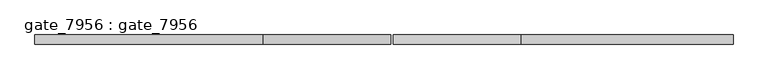
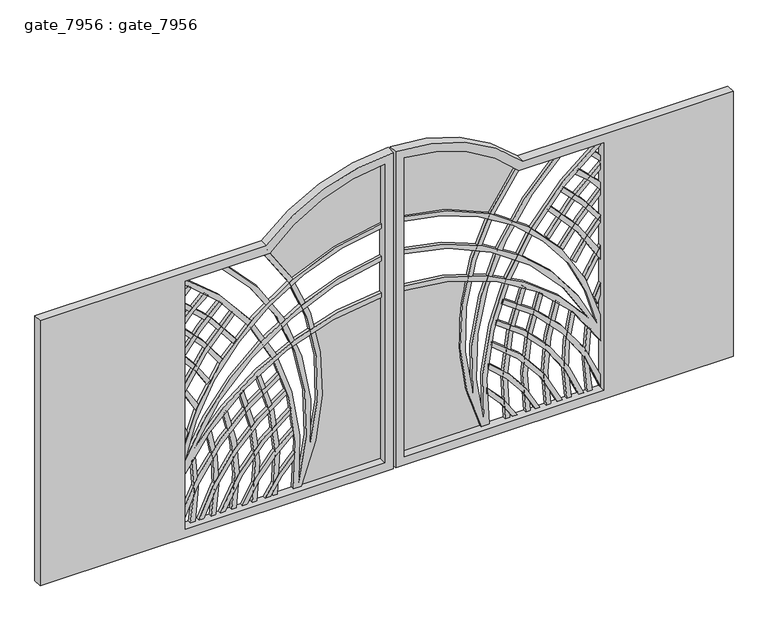
"""IFC4 building model written with IfcOpenShell, lengths in millimetres: proxy geometry, gate_7956 : gate_7956."""

from ifc_helpers import new_model, si_unit, point, frame, frame_2d, origin, place, context, project, spatial, polyline, circle_curve, trimmed, segment, composite_curve, outline, extrude, source, transform, mapped, element, save


def gate_7956_gate_7956_2a423054(model_context):
    return source(origin(), model_context, "Body", "SweptSolid", [
        extrude(outline(composite_curve([segment(polyline([(1574.8, -714.375), (1574.8, -1986.4480277), (0.0, -1986.4480277), (0.0, 0.0), (1879.3736556, 0.0)]), True, "CONTINUOUS"), segment(trimmed(circle_curve(frame_2d((881.859553, 3.175)), 997.5191555), [point((1879.3736556, 0.0))], [point((1574.8, -714.375))], False, "CARTESIAN"), True, "CONTINUOUS")], self_intersect=False), holes=[composite_curve([segment(polyline([(1827.2147875, -47.625), (50.8, -47.625), (50.8, -1171.575), (1524.0, -1171.575), (1524.0, -692.4777911)]), True, "CONTINUOUS"), segment(trimmed(circle_curve(frame_2d((881.859553, 3.175)), 946.7191555), [point((1524.0, -692.4777911))], [point((1827.2147875, -47.625))], True, "CARTESIAN"), True, "CONTINUOUS")], self_intersect=False)]), frame((0.0, -50.8, 0.0), z_axis=(0.0, 1.0, 0.0), x_axis=(0.0, 0.0, 1.0)), (0.0, 0.0, 1.0), 50.8),
        extrude(outline(composite_curve([segment(trimmed(circle_curve(frame_2d((188.1193765, 65.6258097)), 1270.1981582), [point((1453.2587424, -47.625))], [point((475.7606767, -1171.575))], False, "CARTESIAN"), True, "CONTINUOUS"), segment(polyline([(475.7606767, -1171.575), (325.438753, -1171.575)]), True, "CONTINUOUS"), segment(trimmed(circle_curve(frame_2d((-306.470048, -9.2092819)), 1323.0278891), [point((325.438753, -1171.575))], [point((1016.0, -47.625))], True, "CARTESIAN"), True, "CONTINUOUS"), segment(polyline([(1016.0, -47.625), (1042.85139, -47.625)]), True, "CONTINUOUS"), segment(trimmed(circle_curve(frame_2d((-321.9912288, -1.7370637)), 1365.6138095), [point((1042.85139, -47.625))], [point((487.9033995, -1101.269586))], False, "CARTESIAN"), True, "CONTINUOUS"), segment(trimmed(circle_curve(frame_2d((-94.5667128, 101.7568292)), 1336.6166195), [point((487.9033995, -1101.269586))], [point((1233.6761327, -47.625))], True, "CARTESIAN"), True, "CONTINUOUS"), segment(polyline([(1233.6761327, -47.625), (1259.2332506, -47.625)]), True, "CONTINUOUS"), segment(trimmed(circle_curve(frame_2d((-94.5667128, 101.7568292)), 1362.0166195), [point((1259.2332506, -47.625))], [point((428.8390935, -1155.6753295))], False, "CARTESIAN"), True, "CONTINUOUS"), segment(trimmed(circle_curve(frame_2d((188.1193765, 65.6258097)), 1244.7981582), [point((428.8390935, -1155.6753295))], [point((1427.7550927, -47.625))], True, "CARTESIAN"), True, "CONTINUOUS"), segment(polyline([(1427.7550927, -47.625), (1453.2587424, -47.625)]), True, "CONTINUOUS")], self_intersect=False)), frame((0.0, -19.05, 0.0), z_axis=(0.0, 1.0, 0.0), x_axis=(0.0, 0.0, 1.0)), (0.0, 0.0, 1.0), 19.05),
        extrude(outline(composite_curve([segment(trimmed(circle_curve(frame_2d((625.1927136, -1831.8247988)), 1451.1947292), [point((50.8, -499.1436094))], [point((1524.0, -692.4777911))], False, "CARTESIAN"), True, "CONTINUOUS"), segment(polyline([(1524.0, -692.4777911), (1524.0, -717.8616311), (1508.2761961, -712.4096154)]), True, "CONTINUOUS"), segment(trimmed(circle_curve(frame_2d((625.2005352, -1831.8604357)), 1425.8305516), [point((1508.2761961, -712.4096154))], [point((270.5135839, -450.849962))], True, "CARTESIAN"), True, "CONTINUOUS"), segment(trimmed(circle_curve(frame_2d((428.9211986, -1911.4736244)), 1469.1883662), [point((270.5135839, -450.849962))], [point((1524.0, -932.0263955))], False, "CARTESIAN"), True, "CONTINUOUS"), segment(polyline([(1524.0, -932.0263955), (1524.0, -970.5462776)]), True, "CONTINUOUS"), segment(trimmed(circle_curve(frame_2d((434.6192112, -1905.6521568)), 1435.6787622), [point((1524.0, -970.5462776))], [point((79.5169904, -514.5820935))], True, "CARTESIAN"), True, "CONTINUOUS"), segment(trimmed(circle_curve(frame_2d((251.9754674, -2051.8469137)), 1546.9082241), [point((79.5169904, -514.5820935))], [point((1524.0, -1171.575))], False, "CARTESIAN"), True, "CONTINUOUS"), segment(polyline([(1524.0, -1171.575), (1492.986601, -1171.575)]), True, "CONTINUOUS"), segment(trimmed(circle_curve(frame_2d((251.9754674, -2051.8469137)), 1521.5082241), [point((1492.986601, -1171.575))], [point((50.8, -543.6971508))], True, "CARTESIAN"), True, "CONTINUOUS"), segment(polyline([(50.8, -543.6971508), (50.8, -499.1436094)]), True, "CONTINUOUS")], self_intersect=False)), frame((0.0, -19.05, 0.0), z_axis=(0.0, 1.0, 0.0), x_axis=(0.0, 0.0, 1.0)), (0.0, 0.0, 1.0), 19.05),
        extrude(outline(composite_curve([segment(trimmed(circle_curve(frame_2d((-321.9912288, -1.7370636)), 1251.3138095), [point((766.023996, -619.8059275))], [point((122.1545272, -1171.575))], False, "CARTESIAN"), True, "CONTINUOUS"), segment(polyline([(122.1545272, -1171.575), (50.8, -1171.575)]), True, "CONTINUOUS"), segment(trimmed(circle_curve(frame_2d((-329.3476454, 3.2021804)), 1234.7524675), [point((50.8, -1171.575))], [point((741.6413557, -611.2864))], True, "CARTESIAN"), True, "CONTINUOUS"), segment(polyline([(741.6413557, -611.2864), (766.023996, -619.8059275)]), True, "CONTINUOUS")], self_intersect=False)), frame((0.0, -19.05, 0.0), z_axis=(0.0, 1.0, 0.0), x_axis=(0.0, 0.0, 1.0)), (0.0, 0.0, 1.0), 19.05),
        extrude(outline(composite_curve([segment(trimmed(circle_curve(frame_2d((-321.9912288, -1.7370637)), 1137.0138095), [point((654.3216834, -584.5007383))], [point((50.8, -1075.9005069))], False, "CARTESIAN"), True, "CONTINUOUS"), segment(polyline([(50.8, -1075.9005069), (50.8, -1048.9772277)]), True, "CONTINUOUS"), segment(trimmed(circle_curve(frame_2d((-321.9912288, -1.7370637)), 1111.6138095), [point((50.8, -1048.9772277))], [point((628.7552213, -577.7287729))], True, "CARTESIAN"), True, "CONTINUOUS"), segment(polyline([(628.7552213, -577.7287729), (654.3216834, -584.5007383)]), True, "CONTINUOUS")], self_intersect=False)), frame((0.0, -19.05, 0.0), z_axis=(0.0, 1.0, 0.0), x_axis=(0.0, 0.0, 1.0)), (0.0, 0.0, 1.0), 19.05),
        extrude(outline(composite_curve([segment(trimmed(circle_curve(frame_2d((-321.9912288, -1.7370637)), 1022.7138095), [point((536.7182406, -557.2202617))], [point((50.8, -954.0869132))], False, "CARTESIAN"), True, "CONTINUOUS"), segment(polyline([(50.8, -954.0869132), (50.8, -926.7568118)]), True, "CONTINUOUS"), segment(trimmed(circle_curve(frame_2d((-321.9912288, -1.7370637)), 997.3138095), [point((50.8, -926.7568118))], [point((510.8571668, -550.3702604))], True, "CARTESIAN"), True, "CONTINUOUS"), segment(polyline([(510.8571668, -550.3702604), (536.7182406, -557.2202617)]), True, "CONTINUOUS")], self_intersect=False)), frame((0.0, -19.05, 0.0), z_axis=(0.0, 1.0, 0.0), x_axis=(0.0, 0.0, 1.0)), (0.0, 0.0, 1.0), 19.05),
        extrude(outline(composite_curve([segment(trimmed(circle_curve(frame_2d((-321.9912288, -1.7370637)), 908.4138095), [point((410.7722159, -538.6480277))], [point((50.8, -830.134522))], False, "CARTESIAN"), True, "CONTINUOUS"), segment(polyline([(50.8, -830.134522), (50.8, -802.1994847)]), True, "CONTINUOUS"), segment(trimmed(circle_curve(frame_2d((-321.9912288, -1.7370637)), 883.0138095), [point((50.8, -802.1994847))], [point((379.0365912, -538.6480277))], True, "CARTESIAN"), True, "CONTINUOUS"), segment(polyline([(379.0365912, -538.6480277), (410.7722159, -538.6480277)]), True, "CONTINUOUS")], self_intersect=False)), frame((0.0, -19.05, 0.0), z_axis=(0.0, 1.0, 0.0), x_axis=(0.0, 0.0, 1.0)), (0.0, 0.0, 1.0), 19.05),
        extrude(outline(composite_curve([segment(trimmed(circle_curve(frame_2d((-321.9912288, -1.7370637)), 794.1138095), [point((270.5266887, -530.4517881))], [point((50.8, -702.9099683))], False, "CARTESIAN"), True, "CONTINUOUS"), segment(polyline([(50.8, -702.9099683), (50.8, -674.0075603)]), True, "CONTINUOUS"), segment(trimmed(circle_curve(frame_2d((-321.9912288, -1.7370637)), 768.7138095), [point((50.8, -674.0075603))], [point((236.0245963, -530.4517881))], True, "CARTESIAN"), True, "CONTINUOUS"), segment(polyline([(236.0245963, -530.4517881), (270.5266887, -530.4517881)]), True, "CONTINUOUS")], self_intersect=False)), frame((0.0, -19.05, 0.0), z_axis=(0.0, 1.0, 0.0), x_axis=(0.0, 0.0, 1.0)), (0.0, 0.0, 1.0), 19.05),
        extrude(outline(composite_curve([segment(polyline([(1210.9602193, -867.4506933), (1228.939295, -885.429769)]), True, "CONTINUOUS"), segment(trimmed(circle_curve(frame_2d((188.1193765, 65.6258097)), 1409.8981582), [point((1228.939295, -885.429769))], [point((864.245824, -1171.575))], False, "CARTESIAN"), True, "CONTINUOUS"), segment(polyline([(864.245824, -1171.575), (809.5445985, -1171.575)]), True, "CONTINUOUS"), segment(trimmed(circle_curve(frame_2d((188.1193765, 65.6258097)), 1384.4981582), [point((809.5445985, -1171.575))], [point((1210.9602193, -867.4506933))], True, "CARTESIAN"), True, "CONTINUOUS")], self_intersect=False)), frame((0.0, -19.05, 0.0), z_axis=(0.0, 1.0, 0.0), x_axis=(0.0, 0.0, 1.0)), (0.0, 0.0, 1.0), 19.05),
        extrude(outline(composite_curve([segment(polyline([(1295.7670706, -944.0833092), (1313.7464656, -962.0627043)]), True, "CONTINUOUS"), segment(trimmed(circle_curve(frame_2d((298.9547736, -40.580869)), 1370.7410225), [point((1313.7464656, -962.0627043))], [point((1073.4115036, -1171.575))], False, "CARTESIAN"), True, "CONTINUOUS"), segment(polyline([(1073.4115036, -1171.575), (1034.1276953, -1171.575)]), True, "CONTINUOUS"), segment(trimmed(circle_curve(frame_2d((188.1193765, 65.6258097)), 1498.7981582), [point((1034.1276953, -1171.575))], [point((1295.7670706, -944.0833092))], True, "CARTESIAN"), True, "CONTINUOUS")], self_intersect=False)), frame((0.0, -19.05, 0.0), z_axis=(0.0, 1.0, 0.0), x_axis=(0.0, 0.0, 1.0)), (0.0, 0.0, 1.0), 19.05),
        extrude(outline(composite_curve([segment(polyline([(1371.3808408, -1023.8325474), (1393.8084123, -1046.2601189)]), True, "CONTINUOUS"), segment(trimmed(circle_curve(frame_2d((157.0059526, 65.2274597)), 1662.854462), [point((1393.8084123, -1046.2601189))], [point((1268.4935312, -1171.575))], False, "CARTESIAN"), True, "CONTINUOUS"), segment(polyline([(1268.4935312, -1171.575), (1223.2134903, -1171.575)]), True, "CONTINUOUS"), segment(trimmed(circle_curve(frame_2d((881.0604584, -680.2699964)), 598.7063586), [point((1223.2134903, -1171.575))], [point((1371.3808408, -1023.8325474))], True, "CARTESIAN"), True, "CONTINUOUS")], self_intersect=False)), frame((0.0, -19.05, 0.0), z_axis=(0.0, 1.0, 0.0), x_axis=(0.0, 0.0, 1.0)), (0.0, 0.0, 1.0), 19.05),
        extrude(outline(composite_curve([segment(polyline([(1448.1437026, -1116.942791), (1466.2607278, -1135.0598162)]), True, "CONTINUOUS"), segment(trimmed(circle_curve(frame_2d((2369.5144168, -2074.828689)), 1303.469509), [point((1466.2607278, -1135.0598162))], [point((1429.745544, -1171.575))], True, "CARTESIAN"), True, "CONTINUOUS"), segment(polyline([(1429.745544, -1171.575), (1393.6228205, -1171.575)]), True, "CONTINUOUS"), segment(trimmed(circle_curve(frame_2d((2581.8039176, -2302.8138821)), 1640.5717686), [point((1393.6228205, -1171.575))], [point((1448.1437026, -1116.942791))], False, "CARTESIAN"), True, "CONTINUOUS")], self_intersect=False)), frame((0.0, -19.05, 0.0), z_axis=(0.0, 1.0, 0.0), x_axis=(0.0, 0.0, 1.0)), (0.0, 0.0, 1.0), 19.05),
        extrude(outline(composite_curve([segment(polyline([(50.8, -1123.3836365), (50.8, -1096.2682984)]), True, "CONTINUOUS"), segment(trimmed(circle_curve(frame_2d((249.227799, -2294.693819)), 1214.741668), [point((50.8, -1096.2682984))], [point((439.2593722, -1094.9082877))], False, "CARTESIAN"), True, "CONTINUOUS"), segment(polyline([(439.2593722, -1094.9082877), (417.7529701, -1116.4146899)]), True, "CONTINUOUS"), segment(trimmed(circle_curve(frame_2d((251.9754674, -2051.8469137)), 950.0082241), [point((417.7529701, -1116.4146899))], [point((50.8, -1123.3836365))], True, "CARTESIAN"), True, "CONTINUOUS")], self_intersect=False)), frame((0.0, -19.05, 0.0), z_axis=(0.0, 1.0, 0.0), x_axis=(0.0, 0.0, 1.0)), (0.0, 0.0, 1.0), 19.05),
        extrude(outline(composite_curve([segment(polyline([(50.8, -1006.7247069), (50.8, -980.869582)]), True, "CONTINUOUS"), segment(trimmed(circle_curve(frame_2d((251.9754674, -2051.8469137)), 1089.7082241), [point((50.8, -980.869582))], [point((559.4182819, -1006.4078053))], False, "CARTESIAN"), True, "CONTINUOUS"), segment(polyline([(559.4182819, -1006.4078053), (538.8861292, -1026.939958)]), True, "CONTINUOUS"), segment(trimmed(circle_curve(frame_2d((251.9754674, -2051.8469137)), 1064.3082241), [point((538.8861292, -1026.939958))], [point((50.8, -1006.7247069))], True, "CARTESIAN"), True, "CONTINUOUS")], self_intersect=False)), frame((0.0, -19.05, 0.0), z_axis=(0.0, 1.0, 0.0), x_axis=(0.0, 0.0, 1.0)), (0.0, 0.0, 1.0), 19.05),
        extrude(outline(composite_curve([segment(polyline([(50.8, -890.30598), (50.8, -864.7646777)]), True, "CONTINUOUS"), segment(trimmed(circle_curve(frame_2d((251.9754674, -2051.8469137)), 1204.0082241), [point((50.8, -864.7646777))], [point((656.0575932, -917.6716895))], False, "CARTESIAN"), True, "CONTINUOUS"), segment(polyline([(656.0575932, -917.6716895), (636.1282841, -937.6009986)]), True, "CONTINUOUS"), segment(trimmed(circle_curve(frame_2d((249.671635, -2074.7397377)), 1201.0134277), [point((636.1282841, -937.6009986))], [point((50.8, -890.30598))], True, "CARTESIAN"), True, "CONTINUOUS")], self_intersect=False)), frame((0.0, -19.05, 0.0), z_axis=(0.0, 1.0, 0.0), x_axis=(0.0, 0.0, 1.0)), (0.0, 0.0, 1.0), 19.05),
        extrude(outline(composite_curve([segment(polyline([(50.8, -774.6859578), (50.8, -748.9789216)]), True, "CONTINUOUS"), segment(trimmed(circle_curve(frame_2d((251.9754674, -2051.8469137)), 1318.3082241), [point((50.8, -748.9789216))], [point((737.9350335, -826.3756274))], False, "CARTESIAN"), True, "CONTINUOUS"), segment(polyline([(737.9350335, -826.3756274), (718.3335001, -845.9771607)]), True, "CONTINUOUS"), segment(trimmed(circle_curve(frame_2d((251.9754674, -2051.8469137)), 1292.9082241), [point((718.3335001, -845.9771607))], [point((50.8, -774.6859578))], True, "CARTESIAN"), True, "CONTINUOUS")], self_intersect=False)), frame((0.0, -19.05, 0.0), z_axis=(0.0, 1.0, 0.0), x_axis=(0.0, 0.0, 1.0)), (0.0, 0.0, 1.0), 19.05),
        extrude(outline(composite_curve([segment(polyline([(50.8, -659.0930168), (50.8, -633.4341547)]), True, "CONTINUOUS"), segment(trimmed(circle_curve(frame_2d((251.9754674, -2051.8469137)), 1432.6082241), [point((50.8, -633.4341547))], [point((808.380048, -731.7028813))], False, "CARTESIAN"), True, "CONTINUOUS"), segment(polyline([(808.380048, -731.7028813), (788.9599222, -751.1230071)]), True, "CONTINUOUS"), segment(trimmed(circle_curve(frame_2d((251.9754674, -2051.8469137)), 1407.2082241), [point((788.9599222, -751.1230071))], [point((50.8, -659.0930168))], True, "CARTESIAN"), True, "CONTINUOUS")], self_intersect=False)), frame((0.0, -19.05, 0.0), z_axis=(0.0, 1.0, 0.0), x_axis=(0.0, 0.0, 1.0)), (0.0, 0.0, 1.0), 19.05),
        extrude(outline(polyline([(553.3842288, -1150.9205103), (593.450224, -1138.1641492), (672.1451492, -1171.575), (609.2386529, -1171.575), (553.3842288, -1150.9205103)])), frame((0.0, -19.05, 0.0), z_axis=(0.0, 1.0, 0.0), x_axis=(0.0, 0.0, 1.0)), (0.0, 0.0, 1.0), 19.05),
        extrude(outline(composite_curve([segment(trimmed(circle_curve(frame_2d((251.9754673, -2051.8469137)), 1064.3082241), [point((850.2006371, -1171.575))], [point((711.3700205, -1091.7903318))], True, "CARTESIAN"), True, "CONTINUOUS"), segment(polyline([(711.3700205, -1091.7903318), (740.9012216, -1077.980588)]), True, "CONTINUOUS"), segment(trimmed(circle_curve(frame_2d((251.9754674, -2051.8469137)), 1089.7082241), [point((740.9012216, -1077.980588))], [point((894.3035545, -1171.575))], False, "CARTESIAN"), True, "CONTINUOUS"), segment(polyline([(894.3035545, -1171.575), (850.2006371, -1171.575)]), True, "CONTINUOUS")], self_intersect=False)), frame((0.0, -19.05, 0.0), z_axis=(0.0, 1.0, 0.0), x_axis=(0.0, 0.0, 1.0)), (0.0, 0.0, 1.0), 19.05),
        extrude(outline(composite_curve([segment(trimmed(circle_curve(frame_2d((436.5150762, -1780.3292563)), 853.0665783), [point((1034.1276953, -1171.575))], [point((842.2813497, -1029.9451424))], True, "CARTESIAN"), True, "CONTINUOUS"), segment(polyline([(842.2813497, -1029.9451424), (859.7363544, -1012.4901377)]), True, "CONTINUOUS"), segment(trimmed(circle_curve(frame_2d((251.9754673, -2051.8469137)), 1204.0082241), [point((859.7363544, -1012.4901377))], [point((1073.4115036, -1171.575))], False, "CARTESIAN"), True, "CONTINUOUS"), segment(polyline([(1073.4115036, -1171.575), (1034.1276953, -1171.575)]), True, "CONTINUOUS")], self_intersect=False)), frame((0.0, -19.05, 0.0), z_axis=(0.0, 1.0, 0.0), x_axis=(0.0, 0.0, 1.0)), (0.0, 0.0, 1.0), 19.05),
        extrude(outline(composite_curve([segment(polyline([(943.9740273, -959.7161207), (962.3717805, -941.3183675)]), True, "CONTINUOUS"), segment(trimmed(circle_curve(frame_2d((251.9754673, -2051.8469138)), 1318.3082242), [point((962.3717805, -941.3183675))], [point((1233.3306179, -1171.575))], False, "CARTESIAN"), True, "CONTINUOUS"), segment(polyline([(1233.3306179, -1171.575), (1198.9353576, -1171.575)]), True, "CONTINUOUS"), segment(trimmed(circle_curve(frame_2d((251.9754673, -2051.8469138)), 1292.9082241), [point((1198.9353576, -1171.575))], [point((943.9740273, -959.7161207))], True, "CARTESIAN"), True, "CONTINUOUS")], self_intersect=False)), frame((0.0, -19.05, 0.0), z_axis=(0.0, 1.0, 0.0), x_axis=(0.0, 0.0, 1.0)), (0.0, 0.0, 1.0), 19.05),
        extrude(outline(composite_curve([segment(polyline([(1035.0267606, -882.6310833), (1053.3289179, -864.3289261)]), True, "CONTINUOUS"), segment(trimmed(circle_curve(frame_2d((251.9754673, -2051.8469137)), 1432.6082241), [point((1053.3289179, -864.3289261))], [point((1382.2354736, -1171.575))], False, "CARTESIAN"), True, "CONTINUOUS"), segment(polyline([(1382.2354736, -1171.575), (1349.8626855, -1171.575)]), True, "CONTINUOUS"), segment(trimmed(circle_curve(frame_2d((251.9754674, -2051.8469137)), 1407.2082241), [point((1349.8626855, -1171.575))], [point((1035.0267606, -882.6310833))], True, "CARTESIAN"), True, "CONTINUOUS")], self_intersect=False)), frame((0.0, -19.05, 0.0), z_axis=(0.0, 1.0, 0.0), x_axis=(0.0, 0.0, 1.0)), (0.0, 0.0, 1.0), 19.05),
        extrude(outline(composite_curve([segment(trimmed(circle_curve(frame_2d((881.859553, 3.175)), 946.7191555), [point((1827.2147875, -47.625))], [point((1524.0, -692.4777911))], False, "CARTESIAN"), True, "CONTINUOUS"), segment(trimmed(circle_curve(frame_2d((625.1927137, -1831.8247988)), 1451.1947292), [point((1524.0, -692.4777911))], [point((1300.6036994, -547.3847876))], True, "CARTESIAN"), True, "CONTINUOUS"), segment(trimmed(circle_curve(frame_2d((188.1193765, 65.6258097)), 1270.1981582), [point((1300.6036994, -547.3847876))], [point((1453.2587424, -47.625))], True, "CARTESIAN"), True, "CONTINUOUS"), segment(polyline([(1453.2587424, -47.625), (1827.2147875, -47.625)]), True, "CONTINUOUS")], self_intersect=False)), frame((0.0, -6.35, 0.0), z_axis=(0.0, 1.0, 0.0), x_axis=(0.0, 0.0, 1.0)), (0.0, 0.0, 1.0), 6.35),
        extrude(outline(composite_curve([segment(trimmed(circle_curve(frame_2d((-306.470048, -9.2092819)), 1323.0278891), [point((1016.0, -47.625))], [point((951.8602911, -417.8748577))], False, "CARTESIAN"), True, "CONTINUOUS"), segment(trimmed(circle_curve(frame_2d((625.1927136, -1831.8247988)), 1451.1947292), [point((951.8602911, -417.8748577))], [point((50.8, -499.1436094))], True, "CARTESIAN"), True, "CONTINUOUS"), segment(polyline([(50.8, -499.1436094), (50.8, -47.625), (1016.0, -47.625)]), True, "CONTINUOUS")], self_intersect=False)), frame((0.0, -6.35, 0.0), z_axis=(0.0, 1.0, 0.0), x_axis=(0.0, 0.0, 1.0)), (0.0, 0.0, 1.0), 6.35),
        extrude(outline(composite_curve([segment(trimmed(circle_curve(frame_2d((881.859553, 9.525)), 997.5191555), [point((1574.8, 727.075))], [point((1879.3736556, 12.7))], False, "CARTESIAN"), True, "CONTINUOUS"), segment(polyline([(1879.3736556, 12.7), (0.0, 12.7), (0.0, 1910.3857812), (1574.8, 1910.3857812), (1574.8, 727.075)]), True, "CONTINUOUS")], self_intersect=False), holes=[composite_curve([segment(trimmed(circle_curve(frame_2d((881.859553, 9.525)), 946.7191555), [point((1827.2147875, 60.325))], [point((1524.0, 705.1777911))], True, "CARTESIAN"), True, "CONTINUOUS"), segment(polyline([(1524.0, 705.1777911), (1524.0, 1184.275), (50.8, 1184.275), (50.8, 60.325), (1827.2147875, 60.325)]), True, "CONTINUOUS")], self_intersect=False)]), frame((0.0, -50.8, 0.0), z_axis=(0.0, 1.0, 0.0), x_axis=(0.0, 0.0, 1.0)), (0.0, 0.0, 1.0), 50.8),
        extrude(outline(composite_curve([segment(polyline([(1453.2587424, 60.325), (1427.7550927, 60.325)]), True, "CONTINUOUS"), segment(trimmed(circle_curve(frame_2d((188.1193765, -52.9258097)), 1244.7981582), [point((1427.7550927, 60.325))], [point((428.8390935, 1168.3753295))], True, "CARTESIAN"), True, "CONTINUOUS"), segment(trimmed(circle_curve(frame_2d((-94.5667128, -89.0568292)), 1362.0166195), [point((428.8390935, 1168.3753295))], [point((1259.2332506, 60.325))], False, "CARTESIAN"), True, "CONTINUOUS"), segment(polyline([(1259.2332506, 60.325), (1233.6761327, 60.325)]), True, "CONTINUOUS"), segment(trimmed(circle_curve(frame_2d((-94.5667128, -89.0568292)), 1336.6166195), [point((1233.6761327, 60.325))], [point((487.9033995, 1113.969586))], True, "CARTESIAN"), True, "CONTINUOUS"), segment(trimmed(circle_curve(frame_2d((-321.9912288, 14.4370637)), 1365.6138095), [point((487.9033995, 1113.969586))], [point((1042.85139, 60.325))], False, "CARTESIAN"), True, "CONTINUOUS"), segment(polyline([(1042.85139, 60.325), (1016.0, 60.325)]), True, "CONTINUOUS"), segment(trimmed(circle_curve(frame_2d((-306.470048, 21.9092819)), 1323.0278891), [point((1016.0, 60.325))], [point((325.438753, 1184.275))], True, "CARTESIAN"), True, "CONTINUOUS"), segment(polyline([(325.438753, 1184.275), (475.7606767, 1184.275)]), True, "CONTINUOUS"), segment(trimmed(circle_curve(frame_2d((188.1193765, -52.9258097)), 1270.1981582), [point((475.7606767, 1184.275))], [point((1453.2587424, 60.325))], False, "CARTESIAN"), True, "CONTINUOUS")], self_intersect=False)), frame((0.0, -19.05, 0.0), z_axis=(0.0, 1.0, 0.0), x_axis=(0.0, 0.0, 1.0)), (0.0, 0.0, 1.0), 19.05),
        extrude(outline(composite_curve([segment(polyline([(50.8, 511.8436094), (50.8, 556.3971508)]), True, "CONTINUOUS"), segment(trimmed(circle_curve(frame_2d((251.9754674, 2064.5469137)), 1521.5082241), [point((50.8, 556.3971508))], [point((1492.986601, 1184.275))], True, "CARTESIAN"), True, "CONTINUOUS"), segment(polyline([(1492.986601, 1184.275), (1524.0, 1184.275)]), True, "CONTINUOUS"), segment(trimmed(circle_curve(frame_2d((251.9754674, 2064.5469137)), 1546.9082241), [point((1524.0, 1184.275))], [point((79.5169904, 527.2820935))], False, "CARTESIAN"), True, "CONTINUOUS"), segment(trimmed(circle_curve(frame_2d((434.6192112, 1918.3521568)), 1435.6787622), [point((79.5169904, 527.2820935))], [point((1524.0, 983.2462776))], True, "CARTESIAN"), True, "CONTINUOUS"), segment(polyline([(1524.0, 983.2462776), (1524.0, 944.7263955)]), True, "CONTINUOUS"), segment(trimmed(circle_curve(frame_2d((428.9211986, 1924.1736244)), 1469.1883662), [point((1524.0, 944.7263955))], [point((270.5135839, 463.549962))], False, "CARTESIAN"), True, "CONTINUOUS"), segment(trimmed(circle_curve(frame_2d((625.2005352, 1844.5604357)), 1425.8305516), [point((270.5135839, 463.549962))], [point((1508.2761961, 725.1096154))], True, "CARTESIAN"), True, "CONTINUOUS"), segment(polyline([(1508.2761961, 725.1096154), (1524.0, 730.5616311), (1524.0, 705.1777911)]), True, "CONTINUOUS"), segment(trimmed(circle_curve(frame_2d((625.1927136, 1844.5247988)), 1451.1947292), [point((1524.0, 705.1777911))], [point((50.8, 511.8436094))], False, "CARTESIAN"), True, "CONTINUOUS")], self_intersect=False)), frame((0.0, -19.05, 0.0), z_axis=(0.0, 1.0, 0.0), x_axis=(0.0, 0.0, 1.0)), (0.0, 0.0, 1.0), 19.05),
        extrude(outline(composite_curve([segment(polyline([(766.023996, 632.5059275), (741.6413557, 623.9864)]), True, "CONTINUOUS"), segment(trimmed(circle_curve(frame_2d((-329.3476454, 9.4978196)), 1234.7524675), [point((741.6413557, 623.9864))], [point((50.8, 1184.275))], True, "CARTESIAN"), True, "CONTINUOUS"), segment(polyline([(50.8, 1184.275), (122.1545272, 1184.275)]), True, "CONTINUOUS"), segment(trimmed(circle_curve(frame_2d((-321.9912288, 14.4370636)), 1251.3138095), [point((122.1545272, 1184.275))], [point((766.023996, 632.5059275))], False, "CARTESIAN"), True, "CONTINUOUS")], self_intersect=False)), frame((0.0, -19.05, 0.0), z_axis=(0.0, 1.0, 0.0), x_axis=(0.0, 0.0, 1.0)), (0.0, 0.0, 1.0), 19.05),
        extrude(outline(composite_curve([segment(polyline([(654.3216834, 597.2007383), (628.7552213, 590.4287729)]), True, "CONTINUOUS"), segment(trimmed(circle_curve(frame_2d((-321.9912288, 14.4370637)), 1111.6138095), [point((628.7552213, 590.4287729))], [point((50.8, 1061.6772277))], True, "CARTESIAN"), True, "CONTINUOUS"), segment(polyline([(50.8, 1061.6772277), (50.8, 1088.6005069)]), True, "CONTINUOUS"), segment(trimmed(circle_curve(frame_2d((-321.9912288, 14.4370637)), 1137.0138095), [point((50.8, 1088.6005069))], [point((654.3216834, 597.2007383))], False, "CARTESIAN"), True, "CONTINUOUS")], self_intersect=False)), frame((0.0, -19.05, 0.0), z_axis=(0.0, 1.0, 0.0), x_axis=(0.0, 0.0, 1.0)), (0.0, 0.0, 1.0), 19.05),
        extrude(outline(composite_curve([segment(polyline([(536.7182406, 569.9202617), (510.8571668, 563.0702604)]), True, "CONTINUOUS"), segment(trimmed(circle_curve(frame_2d((-321.9912288, 14.4370637)), 997.3138095), [point((510.8571668, 563.0702604))], [point((50.8, 939.4568118))], True, "CARTESIAN"), True, "CONTINUOUS"), segment(polyline([(50.8, 939.4568118), (50.8, 966.7869132)]), True, "CONTINUOUS"), segment(trimmed(circle_curve(frame_2d((-321.9912288, 14.4370637)), 1022.7138095), [point((50.8, 966.7869132))], [point((536.7182406, 569.9202617))], False, "CARTESIAN"), True, "CONTINUOUS")], self_intersect=False)), frame((0.0, -19.05, 0.0), z_axis=(0.0, 1.0, 0.0), x_axis=(0.0, 0.0, 1.0)), (0.0, 0.0, 1.0), 19.05),
        extrude(outline(composite_curve([segment(polyline([(410.7722159, 551.3480277), (379.0365912, 551.3480277)]), True, "CONTINUOUS"), segment(trimmed(circle_curve(frame_2d((-321.9912288, 14.4370637)), 883.0138095), [point((379.0365912, 551.3480277))], [point((50.8, 814.8994847))], True, "CARTESIAN"), True, "CONTINUOUS"), segment(polyline([(50.8, 814.8994847), (50.8, 842.834522)]), True, "CONTINUOUS"), segment(trimmed(circle_curve(frame_2d((-321.9912288, 14.4370637)), 908.4138095), [point((50.8, 842.834522))], [point((410.7722159, 551.3480277))], False, "CARTESIAN"), True, "CONTINUOUS")], self_intersect=False)), frame((0.0, -19.05, 0.0), z_axis=(0.0, 1.0, 0.0), x_axis=(0.0, 0.0, 1.0)), (0.0, 0.0, 1.0), 19.05),
        extrude(outline(composite_curve([segment(polyline([(270.5266887, 543.1517881), (236.0245963, 543.1517881)]), True, "CONTINUOUS"), segment(trimmed(circle_curve(frame_2d((-321.9912288, 14.4370637)), 768.7138095), [point((236.0245963, 543.1517881))], [point((50.8, 686.7075603))], True, "CARTESIAN"), True, "CONTINUOUS"), segment(polyline([(50.8, 686.7075603), (50.8, 715.6099683)]), True, "CONTINUOUS"), segment(trimmed(circle_curve(frame_2d((-321.9912288, 14.4370637)), 794.1138095), [point((50.8, 715.6099683))], [point((270.5266887, 543.1517881))], False, "CARTESIAN"), True, "CONTINUOUS")], self_intersect=False)), frame((0.0, -19.05, 0.0), z_axis=(0.0, 1.0, 0.0), x_axis=(0.0, 0.0, 1.0)), (0.0, 0.0, 1.0), 19.05),
        extrude(outline(composite_curve([segment(trimmed(circle_curve(frame_2d((188.1193765, -52.9258097)), 1384.4981582), [point((1210.9602193, 880.1506933))], [point((809.5445985, 1184.275))], True, "CARTESIAN"), True, "CONTINUOUS"), segment(polyline([(809.5445985, 1184.275), (864.245824, 1184.275)]), True, "CONTINUOUS"), segment(trimmed(circle_curve(frame_2d((188.1193765, -52.9258097)), 1409.8981582), [point((864.245824, 1184.275))], [point((1228.939295, 898.129769))], False, "CARTESIAN"), True, "CONTINUOUS"), segment(polyline([(1228.939295, 898.129769), (1210.9602193, 880.1506933)]), True, "CONTINUOUS")], self_intersect=False)), frame((0.0, -19.05, 0.0), z_axis=(0.0, 1.0, 0.0), x_axis=(0.0, 0.0, 1.0)), (0.0, 0.0, 1.0), 19.05),
        extrude(outline(composite_curve([segment(trimmed(circle_curve(frame_2d((188.1193765, -52.9258097)), 1498.7981582), [point((1295.7670706, 956.7833092))], [point((1034.1276953, 1184.275))], True, "CARTESIAN"), True, "CONTINUOUS"), segment(polyline([(1034.1276953, 1184.275), (1073.4115036, 1184.275)]), True, "CONTINUOUS"), segment(trimmed(circle_curve(frame_2d((298.9547736, 53.280869)), 1370.7410225), [point((1073.4115036, 1184.275))], [point((1313.7464656, 974.7627043))], False, "CARTESIAN"), True, "CONTINUOUS"), segment(polyline([(1313.7464656, 974.7627043), (1295.7670706, 956.7833092)]), True, "CONTINUOUS")], self_intersect=False)), frame((0.0, -19.05, 0.0), z_axis=(0.0, 1.0, 0.0), x_axis=(0.0, 0.0, 1.0)), (0.0, 0.0, 1.0), 19.05),
        extrude(outline(composite_curve([segment(trimmed(circle_curve(frame_2d((881.0604584, 692.9699964)), 598.7063586), [point((1371.3808408, 1036.5325474))], [point((1223.2134903, 1184.275))], True, "CARTESIAN"), True, "CONTINUOUS"), segment(polyline([(1223.2134903, 1184.275), (1268.4935312, 1184.275)]), True, "CONTINUOUS"), segment(trimmed(circle_curve(frame_2d((157.0059526, -52.5274597)), 1662.854462), [point((1268.4935312, 1184.275))], [point((1393.8084123, 1058.9601189))], False, "CARTESIAN"), True, "CONTINUOUS"), segment(polyline([(1393.8084123, 1058.9601189), (1371.3808408, 1036.5325474)]), True, "CONTINUOUS")], self_intersect=False)), frame((0.0, -19.05, 0.0), z_axis=(0.0, 1.0, 0.0), x_axis=(0.0, 0.0, 1.0)), (0.0, 0.0, 1.0), 19.05),
        extrude(outline(composite_curve([segment(trimmed(circle_curve(frame_2d((2581.8039176, 2315.5138821)), 1640.5717686), [point((1448.1437026, 1129.642791))], [point((1393.6228205, 1184.275))], False, "CARTESIAN"), True, "CONTINUOUS"), segment(polyline([(1393.6228205, 1184.275), (1429.745544, 1184.275)]), True, "CONTINUOUS"), segment(trimmed(circle_curve(frame_2d((2369.5144168, 2087.528689)), 1303.469509), [point((1429.745544, 1184.275))], [point((1466.2607278, 1147.7598162))], True, "CARTESIAN"), True, "CONTINUOUS"), segment(polyline([(1466.2607278, 1147.7598162), (1448.1437026, 1129.642791)]), True, "CONTINUOUS")], self_intersect=False)), frame((0.0, -19.05, 0.0), z_axis=(0.0, 1.0, 0.0), x_axis=(0.0, 0.0, 1.0)), (0.0, 0.0, 1.0), 19.05),
        extrude(outline(composite_curve([segment(trimmed(circle_curve(frame_2d((251.9754674, 2064.5469137)), 950.0082241), [point((50.8, 1136.0836365))], [point((417.7529701, 1129.1146899))], True, "CARTESIAN"), True, "CONTINUOUS"), segment(polyline([(417.7529701, 1129.1146899), (439.2593722, 1107.6082877)]), True, "CONTINUOUS"), segment(trimmed(circle_curve(frame_2d((249.227799, 2307.393819)), 1214.741668), [point((439.2593722, 1107.6082877))], [point((50.8, 1108.9682984))], False, "CARTESIAN"), True, "CONTINUOUS"), segment(polyline([(50.8, 1108.9682984), (50.8, 1136.0836365)]), True, "CONTINUOUS")], self_intersect=False)), frame((0.0, -19.05, 0.0), z_axis=(0.0, 1.0, 0.0), x_axis=(0.0, 0.0, 1.0)), (0.0, 0.0, 1.0), 19.05),
        extrude(outline(composite_curve([segment(trimmed(circle_curve(frame_2d((251.9754674, 2064.5469137)), 1064.3082241), [point((50.8, 1019.4247069))], [point((538.8861292, 1039.639958))], True, "CARTESIAN"), True, "CONTINUOUS"), segment(polyline([(538.8861292, 1039.639958), (559.4182819, 1019.1078053)]), True, "CONTINUOUS"), segment(trimmed(circle_curve(frame_2d((251.9754674, 2064.5469137)), 1089.7082241), [point((559.4182819, 1019.1078053))], [point((50.8, 993.569582))], False, "CARTESIAN"), True, "CONTINUOUS"), segment(polyline([(50.8, 993.569582), (50.8, 1019.4247069)]), True, "CONTINUOUS")], self_intersect=False)), frame((0.0, -19.05, 0.0), z_axis=(0.0, 1.0, 0.0), x_axis=(0.0, 0.0, 1.0)), (0.0, 0.0, 1.0), 19.05),
        extrude(outline(composite_curve([segment(trimmed(circle_curve(frame_2d((249.671635, 2087.4397377)), 1201.0134277), [point((50.8, 903.00598))], [point((636.1282841, 950.3009986))], True, "CARTESIAN"), True, "CONTINUOUS"), segment(polyline([(636.1282841, 950.3009986), (656.0575932, 930.3716895)]), True, "CONTINUOUS"), segment(trimmed(circle_curve(frame_2d((251.9754674, 2064.5469137)), 1204.0082241), [point((656.0575932, 930.3716895))], [point((50.8, 877.4646777))], False, "CARTESIAN"), True, "CONTINUOUS"), segment(polyline([(50.8, 877.4646777), (50.8, 903.00598)]), True, "CONTINUOUS")], self_intersect=False)), frame((0.0, -19.05, 0.0), z_axis=(0.0, 1.0, 0.0), x_axis=(0.0, 0.0, 1.0)), (0.0, 0.0, 1.0), 19.05),
        extrude(outline(composite_curve([segment(trimmed(circle_curve(frame_2d((251.9754674, 2064.5469137)), 1292.9082241), [point((50.8, 787.3859578))], [point((718.3335001, 858.6771607))], True, "CARTESIAN"), True, "CONTINUOUS"), segment(polyline([(718.3335001, 858.6771607), (737.9350335, 839.0756274)]), True, "CONTINUOUS"), segment(trimmed(circle_curve(frame_2d((251.9754674, 2064.5469137)), 1318.3082241), [point((737.9350335, 839.0756274))], [point((50.8, 761.6789216))], False, "CARTESIAN"), True, "CONTINUOUS"), segment(polyline([(50.8, 761.6789216), (50.8, 787.3859578)]), True, "CONTINUOUS")], self_intersect=False)), frame((0.0, -19.05, 0.0), z_axis=(0.0, 1.0, 0.0), x_axis=(0.0, 0.0, 1.0)), (0.0, 0.0, 1.0), 19.05),
        extrude(outline(composite_curve([segment(trimmed(circle_curve(frame_2d((251.9754674, 2064.5469137)), 1407.2082241), [point((50.8, 671.7930168))], [point((788.9599222, 763.8230071))], True, "CARTESIAN"), True, "CONTINUOUS"), segment(polyline([(788.9599222, 763.8230071), (808.380048, 744.4028813)]), True, "CONTINUOUS"), segment(trimmed(circle_curve(frame_2d((251.9754674, 2064.5469137)), 1432.6082241), [point((808.380048, 744.4028813))], [point((50.8, 646.1341547))], False, "CARTESIAN"), True, "CONTINUOUS"), segment(polyline([(50.8, 646.1341547), (50.8, 671.7930168)]), True, "CONTINUOUS")], self_intersect=False)), frame((0.0, -19.05, 0.0), z_axis=(0.0, 1.0, 0.0), x_axis=(0.0, 0.0, 1.0)), (0.0, 0.0, 1.0), 19.05),
        extrude(outline(polyline([(553.3842288, 1163.6205103), (609.2386529, 1184.275), (672.1451492, 1184.275), (593.450224, 1150.8641492), (553.3842288, 1163.6205103)])), frame((0.0, -19.05, 0.0), z_axis=(0.0, 1.0, 0.0), x_axis=(0.0, 0.0, 1.0)), (0.0, 0.0, 1.0), 19.05),
        extrude(outline(composite_curve([segment(polyline([(850.2006371, 1184.275), (894.3035545, 1184.275)]), True, "CONTINUOUS"), segment(trimmed(circle_curve(frame_2d((251.9754674, 2064.5469137)), 1089.7082241), [point((894.3035545, 1184.275))], [point((740.9012216, 1090.680588))], False, "CARTESIAN"), True, "CONTINUOUS"), segment(polyline([(740.9012216, 1090.680588), (711.3700205, 1104.4903318)]), True, "CONTINUOUS"), segment(trimmed(circle_curve(frame_2d((251.9754673, 2064.5469137)), 1064.3082241), [point((711.3700205, 1104.4903318))], [point((850.2006371, 1184.275))], True, "CARTESIAN"), True, "CONTINUOUS")], self_intersect=False)), frame((0.0, -19.05, 0.0), z_axis=(0.0, 1.0, 0.0), x_axis=(0.0, 0.0, 1.0)), (0.0, 0.0, 1.0), 19.05),
        extrude(outline(composite_curve([segment(polyline([(1034.1276953, 1184.275), (1073.4115036, 1184.275)]), True, "CONTINUOUS"), segment(trimmed(circle_curve(frame_2d((251.9754673, 2064.5469137)), 1204.0082241), [point((1073.4115036, 1184.275))], [point((859.7363544, 1025.1901377))], False, "CARTESIAN"), True, "CONTINUOUS"), segment(polyline([(859.7363544, 1025.1901377), (842.2813497, 1042.6451424)]), True, "CONTINUOUS"), segment(trimmed(circle_curve(frame_2d((436.5150762, 1793.0292563)), 853.0665783), [point((842.2813497, 1042.6451424))], [point((1034.1276953, 1184.275))], True, "CARTESIAN"), True, "CONTINUOUS")], self_intersect=False)), frame((0.0, -19.05, 0.0), z_axis=(0.0, 1.0, 0.0), x_axis=(0.0, 0.0, 1.0)), (0.0, 0.0, 1.0), 19.05),
        extrude(outline(composite_curve([segment(trimmed(circle_curve(frame_2d((251.9754673, 2064.5469138)), 1292.9082241), [point((943.9740273, 972.4161207))], [point((1198.9353576, 1184.275))], True, "CARTESIAN"), True, "CONTINUOUS"), segment(polyline([(1198.9353576, 1184.275), (1233.3306179, 1184.275)]), True, "CONTINUOUS"), segment(trimmed(circle_curve(frame_2d((251.9754673, 2064.5469138)), 1318.3082242), [point((1233.3306179, 1184.275))], [point((962.3717805, 954.0183675))], False, "CARTESIAN"), True, "CONTINUOUS"), segment(polyline([(962.3717805, 954.0183675), (943.9740273, 972.4161207)]), True, "CONTINUOUS")], self_intersect=False)), frame((0.0, -19.05, 0.0), z_axis=(0.0, 1.0, 0.0), x_axis=(0.0, 0.0, 1.0)), (0.0, 0.0, 1.0), 19.05),
        extrude(outline(composite_curve([segment(trimmed(circle_curve(frame_2d((251.9754674, 2064.5469137)), 1407.2082241), [point((1035.0267606, 895.3310833))], [point((1349.8626855, 1184.275))], True, "CARTESIAN"), True, "CONTINUOUS"), segment(polyline([(1349.8626855, 1184.275), (1382.2354736, 1184.275)]), True, "CONTINUOUS"), segment(trimmed(circle_curve(frame_2d((251.9754673, 2064.5469137)), 1432.6082241), [point((1382.2354736, 1184.275))], [point((1053.3289179, 877.0289261))], False, "CARTESIAN"), True, "CONTINUOUS"), segment(polyline([(1053.3289179, 877.0289261), (1035.0267606, 895.3310833)]), True, "CONTINUOUS")], self_intersect=False)), frame((0.0, -19.05, 0.0), z_axis=(0.0, 1.0, 0.0), x_axis=(0.0, 0.0, 1.0)), (0.0, 0.0, 1.0), 19.05),
        extrude(outline(composite_curve([segment(polyline([(1827.2147875, 60.325), (1453.2587424, 60.325)]), True, "CONTINUOUS"), segment(trimmed(circle_curve(frame_2d((188.1193765, -52.9258097)), 1270.1981582), [point((1453.2587424, 60.325))], [point((1300.6036994, 560.0847876))], True, "CARTESIAN"), True, "CONTINUOUS"), segment(trimmed(circle_curve(frame_2d((625.1927137, 1844.5247988)), 1451.1947292), [point((1300.6036994, 560.0847876))], [point((1524.0, 705.1777911))], True, "CARTESIAN"), True, "CONTINUOUS"), segment(trimmed(circle_curve(frame_2d((881.859553, 9.525)), 946.7191555), [point((1524.0, 705.1777911))], [point((1827.2147875, 60.325))], False, "CARTESIAN"), True, "CONTINUOUS")], self_intersect=False)), frame((0.0, -6.35, 0.0), z_axis=(0.0, 1.0, 0.0), x_axis=(0.0, 0.0, 1.0)), (0.0, 0.0, 1.0), 6.35),
        extrude(outline(composite_curve([segment(polyline([(1016.0, 60.325), (50.8, 60.325), (50.8, 511.8436094)]), True, "CONTINUOUS"), segment(trimmed(circle_curve(frame_2d((625.1927136, 1844.5247988)), 1451.1947292), [point((50.8, 511.8436094))], [point((951.8602911, 430.5748577))], True, "CARTESIAN"), True, "CONTINUOUS"), segment(trimmed(circle_curve(frame_2d((-306.470048, 21.9092819)), 1323.0278891), [point((951.8602911, 430.5748577))], [point((1016.0, 60.325))], False, "CARTESIAN"), True, "CONTINUOUS")], self_intersect=False)), frame((0.0, -6.35, 0.0), z_axis=(0.0, 1.0, 0.0), x_axis=(0.0, 0.0, 1.0)), (0.0, 0.0, 1.0), 6.35),
    ])


if __name__ == "__main__":
    model = new_model("IFC4")
    model_context = context("Model", 3, world=origin())
    ifc_project = project(units=[si_unit("LENGTHUNIT", "METRE", prefix="MILLI")], contexts=[model_context])
    site = spatial("IfcSite", under=ifc_project)
    building = spatial("IfcBuilding", under=site)
    placement = place(None, origin())
    gate_7956_gate_7956_shape = gate_7956_gate_7956_2a423054(model_context)
    element("IfcBuildingElementProxy", 1, Name="gate_7956 : gate_7956", ObjectType="gate_7956 : gate_7956", at=placement, inside=building, context=model_context, shape_type="MappedRepresentation", body=[
        mapped(gate_7956_gate_7956_shape, transform((0.0, 0.0, 0.0), x_axis=(1.0, 0.0, 0.0), y_axis=(0.0, 1.0, 0.0), z_axis=(0.0, 0.0, 1.0))),
    ])
    save(model, "model.ifc")

# Revit data of these elements
# Type "gate_7956 : gate_7956"
#   m.s. sheet = none
#   2" x2" pipe = none
#   1"x1"pipe = none
#   Default Elevation = 0
